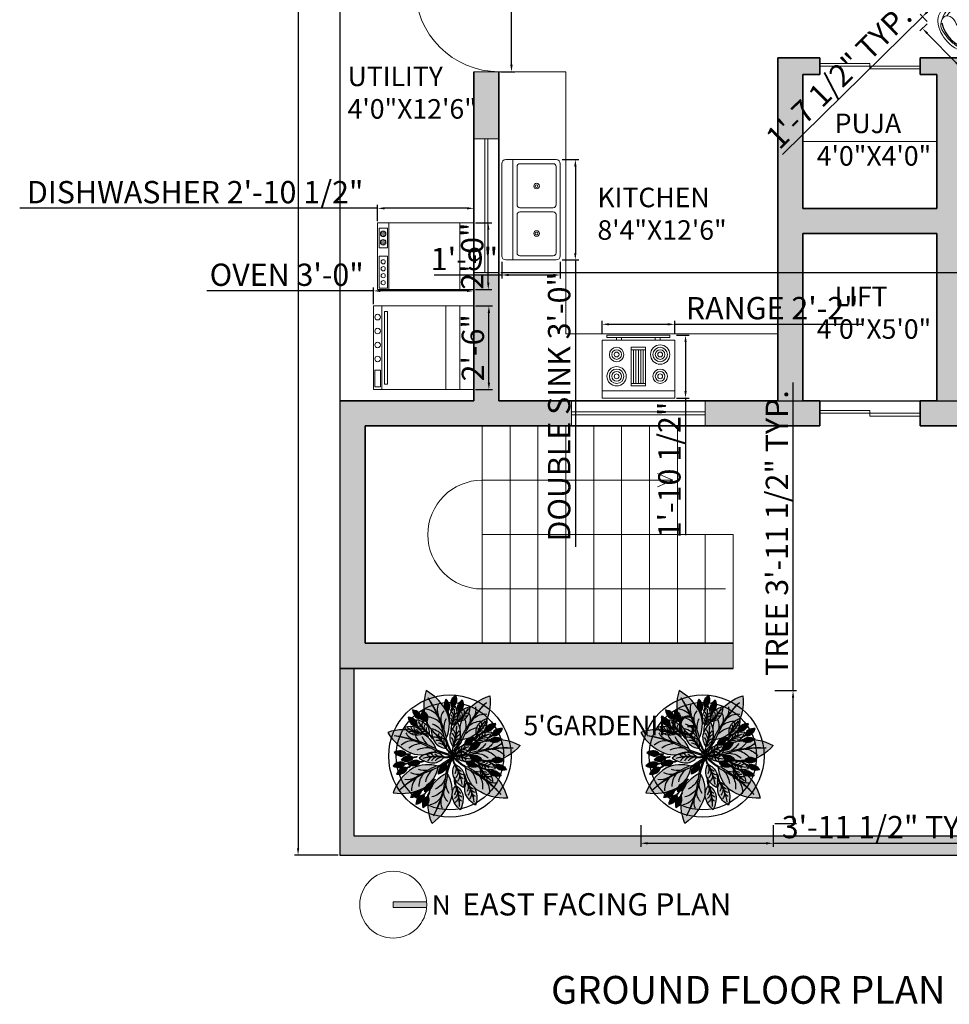
# Model space of a CAD drawing. Units: inches. Extents: x 2700 to 4052, y 1030 to 1872.
# Tile 1 of 8: x 2700 to 3033, y 1048 to 1401. Entities that reach past the tile are written whole.
import ezdxf

# ---------------------------------------------------------------- set-up
doc = ezdxf.new("R2010")
doc.units = ezdxf.units.IN
for name, color, linetype, lineweight in [('A-ANNO-DIMS', 2, 'Continuous', 13), ('A-ANNO-SYMB', 7, 'Continuous', 18), ('A-ANNO-TITL', 7, 'Continuous', 25), ('A-AREA-IDEN', 7, 'Continuous', 18), ('A-DOOR', 4, 'Continuous', 18), ('A-EQPM', 8, 'Continuous', 18), ('A-FLOR-CASE', 8, 'Continuous', 18), ('A-FLOR-FIXT', 9, 'Continuous', 18), ('A-FLOR-STRS', 7, 'Continuous', 18), ('A-FURN', 8, 'Continuous', 18), ('A-GLAZ', 4, 'Continuous', 18), ('A-WALL', 7, 'Continuous', 35), ('A-WALL-PATT', 7, 'Continuous', 13), ('C-PROP', 7, 'Continuous', 25), ('L-PLNT', 3, 'Continuous', 13)]:
    doc.layers.add(name, color=color, linetype=linetype, lineweight=lineweight)
doc.layers.add('C-SITE-PATT', color=252, linetype='Continuous', lineweight=13, true_color=0x939598)
doc.layers.add('IFF-FURN-DETAIL', color=250, linetype='Continuous')
doc.layers.add('MESA', color=7, linetype='Continuous')
doc.styles.get("Standard").update_dxf_attribs({"font": 'arial.ttf'})
doc.dimstyles.new('ISO-25', dxfattribs={"dimtxt": 8, "dimasz": 2.5, "dimexe": 1.25, "dimexo": 0.625, "dimtad": 1, "dimdec": 1, "dimlunit": 3, "dimtxsty": 'Standard', "dimcen": 2.5, "dimclrt": 1, "dimadec": 0, "dimazin": 0, "dimtfac": 1, "dimtdec": 1, "dimtmove": 0, "dimatfit": 3, "dimfxl": 1, "dimarcsym": 0})

# ---------------------------------------------------------------- blocks, each defined once
blk = doc.blocks.new('ILNG95')
for points in [[(120, 308, -0.32971), (51, 384, -0.036099), (50, 422, -0.497733), (75, 439, -0.070621), (96, 429, 0.101868), (133, 414, 0.091794), (259, 412, 0.024114), (351, 433, -0.090294), (638, 458, -0.132412), (775, 407, -0.068618), (816, 368, -0.184346), (943, 0, 1.803905)], [(120, 308, 0.138132), (244, 313, 0.001085), (325, 339, -0.034227), (462, 375, -0.033255), (567, 387, -0.137428), (727, 350, -4.561553)], [(120, 308, 0.138132), (244, 313, 0.001085), (325, 339, -0.034227), (462, 375, -0.033255), (567, 387, -0.137428), (727, 350, -4.561553)], [(235, 308, 0.064243), (394, 307, 0.04414), (433, 315, -0.118032), (643, 329, -6.296816)], [(235, 308, 0.064243), (394, 307, 0.04414), (433, 315, -0.118032), (643, 329, -6.296816)], [(639, 0, 0.078302), (612, 161, -0.233633), (633, 315, -0.28763), (710, 349, -0.317923), (875, 193, -0.032882), (900, 0, 1.140397)], [(639, 0, 0.078302), (612, 161, -0.233633), (633, 315, -0.28763), (710, 349, -0.317923), (875, 193, -0.032882), (900, 0, 1.140397)], [(120, -308, 0.32971), (51, -384, 0.036099), (50, -422, 0.497733), (75, -439, 0.070621), (96, -429, -0.101868), (133, -414, -0.091794), (259, -412, -0.024114), (351, -433, 0.090294), (638, -458, 0.132412), (775, -407, 0.068618), (816, -368, 0.184346), (943, 0, -1.803905)], [(639, 0, -0.078302), (612, -161, 0.233633), (633, -315, 0.28763), (710, -349, 0.317923), (875, -193, 0.032882), (900, 0, -1.140397)], [(639, 0, -0.078302), (612, -161, 0.233633), (633, -315, 0.28763), (710, -349, 0.317923), (875, -193, 0.032882), (900, 0, -1.140397)], [(120, -308, -0.138132), (244, -313, -0.001085), (325, -339, 0.034227), (462, -375, 0.033255), (567, -387, 0.137428), (727, -350, 4.561553)], [(120, -308, -0.138132), (244, -313, -0.001085), (325, -339, 0.034227), (462, -375, 0.033255), (567, -387, 0.137428), (727, -350, 4.561553)], [(235, -308, -0.064243), (394, -307, -0.04414), (433, -315, 0.118032), (643, -329, 6.296816)], [(235, -308, -0.064243), (394, -307, -0.04414), (433, -315, 0.118032), (643, -329, 6.296816)]]:
    blk.add_lwpolyline(points, format="xyb")
blk.add_arc((759, 1), 709, 154.3281, 205.801)
at = {"layer": 'IFF-FURN-DETAIL'}
blk.add_arc((326, -2), 549, 326.8997, 34.6691, dxfattribs=at)
blk.add_arc((326, -2), 549, 326.8997, 34.6691, dxfattribs=at)
blk = doc.blocks.new('Range-Oven - 30 in top')
for p, q in [((0, -3), (30, -3)), ((12, -6), (18, -6)), ((13, -20), (13, -6)), ((14, -6), (14, -20)), ((15, -20), (15, -6)), ((16, -6), (16, -20)), ((17, -20), (17, -6)), ((18, -20), (12, -20)), ((6, -24), (6, -25)), ((8, -25), (8, -24)), ((22, -25), (22, -24)), ((24, -24), (24, -25))]:
    blk.add_line(p, q)
for points in [[(0, -24), (0, 0), (30, 0), (30, -24)], [(12, -21), (12, -5), (18, -5), (18, -21)], [(2, -26), (2, -25), (28, -25), (28, -26)]]:
    blk.add_lwpolyline(points, close=True)
for centre, radius in [((6, -9), 4), ((6, -9), 3), ((6, -9), 2), ((6, -9), 1), ((24, -9), 3), ((24, -9), 2), ((24, -9), 1), ((6, -18), 3), ((6, -18), 2), ((24, -18), 4), ((24, -18), 3), ((24, -18), 2), ((6, -18), 1), ((24, -18), 1)]:
    blk.add_circle(centre, radius)
blk = doc.blocks.new('Sink-double - 36 in top')
for p, q in [((-18, -4), (18, -4)), ((-0.75, -18.5), (-0.75, -6.5)), ((0.75, -6.5), (0.75, -18.5))]:
    blk.add_line(p, q)
for points in [[(-16.5, 0), (16.5, 0)], [(-18, -19.5), (-18, -1.5)], [(18, -1.5), (18, -19.5)], [(-16.5, -18.5), (-16.5, -6.5)], [(-15.5, -5.5), (-1.75, -5.5)], [(1.75, -5.5), (15.5, -5.5)], [(16.5, -6.5), (16.5, -18.5)], [(16.5, -21), (-16.5, -21)], [(-1.75, -19.5), (-15.5, -19.5)], [(15.5, -19.5), (1.75, -19.5)]]:
    blk.add_lwpolyline(points)
for centre, radius in [((-8.5, -12.5), 1), ((-8.5, -12.5), 0.5), ((8.5, -12.5), 1), ((8.5, -12.5), 0.5)]:
    blk.add_circle(centre, radius)
for centre, radius, start, end in [((-16.5, -1.5), 1.5, 90, 180), ((16.5, -1.5), 1.5, 0, 90), ((-15.5, -6.5), 1, 90, 180), ((-1.75, -6.5), 1, 0, 90), ((1.75, -6.5), 1, 90, 180), ((15.5, -6.5), 1, 0, 90), ((-16.5, -19.5), 1.5, 180, 270), ((-15.5, -18.5), 1, 180, 270), ((-1.75, -18.5), 1, 270, 0), ((1.75, -18.5), 1, 180, 270), ((15.5, -18.5), 1, 270, 0), ((16.5, -19.5), 1.5, 270, 0)]:
    blk.add_arc(centre, radius, start, end)
blk = doc.blocks.new('Range-Oven - 30 in front')
for p, q in [((0, 33.00005), (30, 33.00005)), ((30, 10), (0, 10)), ((0, 5), (30, 5))]:
    blk.add_line(p, q)
for points in [[(0, 0), (0, 36.00005), (30, 36.00005), (30, 0)], [(1, 33.50005), (1, 35.50005), (7, 35.50005), (7, 33.50005)], [(2, 31.00005), (2, 32.00005), (28, 32.00005), (28, 31.00005)]]:
    blk.add_lwpolyline(points, close=True)
for centre in [(11, 34.50005), (16, 34.50005), (21, 34.50005), (26, 34.50005)]:
    blk.add_circle(centre, 1)
blk = doc.blocks.new('Dishwasher')
for p, q in [((16, 32.5), (16.75, 32.5)), ((16.5, 32), (16.2942, 31.7942)), ((16.3156, 33.1843), (16.5, 33)), ((17, 32.75), (17, 33.5)), ((17, 32.25), (17, 31.5)), ((18, 32.5), (17.25, 32.5)), ((17.5, 33), (17.6938, 33.1938)), ((17.7061, 31.7939), (17.5, 32)), ((19, 32.5), (19.75, 32.5)), ((19.5, 32), (19.2942, 31.7942)), ((19.3156, 33.1843), (19.5, 33)), ((20, 32.75), (20, 33.5)), ((20, 32.25), (20, 31.5)), ((21, 32.5), (20.25, 32.5)), ((20.5, 33), (20.6938, 33.1938)), ((20.7061, 31.7939), (20.5, 32)), ((24, 30.5), (0, 30.5)), ((0, 5), (24, 5))]:
    blk.add_line(p, q)
for points in [[(0, 0), (0, 34.5), (24, 34.5), (24, 0)], [(0.5, 31), (0.5, 34), (12, 34), (12, 31)], [(15, 31), (15, 34), (22, 34), (22, 31)]]:
    blk.add_lwpolyline(points, close=True)
for centre, radius in [((2.5, 32.5), 0.75), ((5, 32.5), 0.75), ((7.5, 32.5), 0.75), ((10, 32.5), 0.75), ((17, 32.5), 1), ((20, 32.5), 1)]:
    blk.add_circle(centre, radius)
blk = doc.blocks.new('folha Ant')
at = {"layer": 'MESA', "ltscale": 0.8}
h = blk.add_hatch(color=256, dxfattribs=at)
h.dxf.hatch_style = 1
h.set_gradient(color1=(103, 159, 96), color2=(179, 207, 175), one_color=1, tint=0.75, name='INVCURVED')
h.paths.add_polyline_path([(0.2266, 0.0676, 0.199512), (0.0989, 0.0067, 0.09675), (0.3533, 0.0075, -0.086654), (0.1023, -0.0053, 0.192489), (0.2266, -0.0624, 0.158608), (0.3953, 0.0026, 0.158608)])
h = blk.add_hatch(color=256, dxfattribs=at)
h.dxf.hatch_style = 1
h.set_gradient(color1=(179, 116, 77), color2=(114, 74, 49), one_color=1, tint=0.32, name='CURVED')
h.paths.add_polyline_path([(0.05, -0.0003), (0.0485, 0.0057, 0.033108), (0, 0, 0.809082), (0.002, -0.006, -0.032777)])
h.paths.add_polyline_path([(0.0973, 0.0049, 0.033108), (0.0485, 0.0057), (0.05, -0.0003, -0.032777), (0.0983, -0.001), (0.0953, 0.0026)])
h = blk.add_hatch(color=256, dxfattribs=at)
h.dxf.hatch_style = 1
h.set_gradient(color1=(103, 159, 96), color2=(52, 80, 48), one_color=1, tint=0.25)
h.paths.add_polyline_path([(0.3533, 0.0075, -0.09675), (0.0989, 0.0067, 0.007527), (0.0953, 0.0026, 0.014292), (0.1023, -0.0053, 0.086654)])
blk.add_lwpolyline([(0.0983, -0.001), (0.0953, 0.0026), (0.0973, 0.0049, 0.066288), (0, 0, 0.809082), (0.002, -0.006, -0.065625)], format="xyb", close=True, dxfattribs=at)
for centre, radius, start, end in [((0.2359, -0.1164), 0.1842, 92.9121, 139.7695), ((0.211, -0.2242), 0.2922, 50.9055, 86.9554), ((0.2359, 0.1215), 0.1842, 220.2305, 267.0879), ((0.2242, 0.6583), 0.6635, 259.119, 281.2235), ((0.1912, 0.7199), 0.7306, 263.0097, 282.8199), ((0.1144, 0.1192), 0.1187, 277.6411, 318.482), ((0.1515, 0.1013), 0.1129, 290.5634, 330.4539), ((0.211, 0.2293), 0.2922, 273.0446, 309.0945), ((0.2123, 0.0879), 0.0955, 283.0013, 333.1911), ((0.1127, -0.1239), 0.1214, 41.7528, 70.1061), ((0.1853, -0.0821), 0.0727, 27.7376, 79.2347), ((0.2381, -0.0995), 0.0902, 48.8027, 88.011)]:
    blk.add_arc(centre, radius, start, end, dxfattribs=at)
blk = doc.blocks.new('arvore L')
at = {"layer": 'MESA', "ltscale": 0.8}
for radius in [0.35, 0.3077]:
    blk.add_circle((-0.0174, -0.0123), radius, dxfattribs=at)
at = {"layer": 'MESA'}
for p, rotation in [((-0.0038, -0.0034), 111.8634939329907), ((-0.0015, -0.0116), 159.7023978146411), ((-0.002, -0.0223), 210.0932896211622)]:
    blk.add_blockref('folha Ant', p, dxfattribs=dict(at, rotation=rotation))
at = {"layer": 'MESA', "xscale": -1}
for p, rotation in [((-0.0038, 0.0015), 237.4553048776787), ((-0.0054, -0.0158), 189.5771815307885), ((-0.0065, -0.0187), 73.74235818062448), ((-0.0036, -0.0152), 143.2116612097536)]:
    blk.add_blockref('folha Ant', p, dxfattribs=dict(at, rotation=rotation))
at = {"layer": 'MESA'}
for p, xscale, yscale, zscale, rotation in [((-0.0106, 0.2458), -0.2372171158460138, 0.2372171158460219, 0.2372171158460401, 254.670727296299), ((-0.0228, 0.2207), 0.2372171158460145, 0.2372171158460145, 0.2372171158460145, 100.7442899234288), ((0.0048, 0.1582), 0.3672988726102984, 0.3672988726102984, 0.3672988726102984, 49.45009658216958), ((0.0276, 0.2187), -0.2372171158460138, 0.2372171158460219, 0.2372171158460401, 254.670727296299), ((-0.1648, 0.1856), 0.2372171158460308, 0.2372171158460308, 0.2372171158460308, 134.9461414081513), ((-0.1441, 0.1612), -0.2372171158460326, 0.2372171158460219, 0.2372171158460401, 288.8725787810177), ((-0.0127, 0.1293), 0.367298872610303, 0.367298872610303, 0.367298872610303, 78.9591877781593), ((-0.1408, 0.1026), -0.3672988726103232, 0.3672988726103199, 0.3672988726103326, 340.1667721222815), ((-0.189, 0.1454), 0.2372171158460308, 0.2372171158460308, 0.2372171158460308, 134.9461414081513), ((-0.1144, 0.0854), -0.3672988726103342, 0.3672988726103199, 0.3672988726103326, 310.6576809262878), ((-0.0068, -0.0029), 0.4722192998870434, 0.4722192998870434, 0.4722192998870434, 78.95918777814883), ((0.1186, 0.0777), -0.3672988726103297, 0.3672988726103199, 0.3672988726103326, 240.0025576387842), ((0.1681, 0.1193), 0.2372171158460773, 0.2372171158460773, 0.2372171158460773, 34.78192692463861), ((-0.0091, -0.003), 0.4722192998870449, 0.4722192998870449, 0.4722192998870449, 127.7597565182155), ((0.0972, 0.0516), -0.3672988726102771, 0.3672988726103199, 0.3672988726103326, 210.4934664427891), ((0.2063, 0.0923), 0.2372171158460773, 0.2372171158460773, 0.2372171158460773, 34.78192692463861), ((-0.0206, -0.0213), -0.3672988726102771, 0.3672988726103199, 0.3672988726103326, 210.4934664427891), ((0.0473, 0.041), 0.2372171158460773, 0.2372171158460773, 0.2372171158460773, 34.78192692463861), ((0.0807, 0.0116), 0.2372171158460773, 0.2372171158460773, 0.2372171158460773, 34.78192692463861), ((0.1867, 0.0725), -0.237217115846069, 0.2372171158460219, 0.2372171158460401, 188.7083642975024), ((-0.2438, -0.0026), 0.2372171158460885, 0.2372171158460885, 0.2372171158460885, 173.1881796188063), ((-0.0061, -0.0164), 0.4722192998870134, 0.4722192998870134, 0.4722192998870134, 181.8145453364702), ((-0.0239, 0.0106), 0.3672988726102808, 0.3672988726102808, 0.3672988726102808, 341.2516722292817), ((0.082, -0.001), -0.2372171158460231, 0.2372171158460219, 0.2372171158460401, 156.9632117474216), ((-0.2506, -0.0512), 0.2372171158460153, 0.2372171158460153, 0.2372171158460153, 190.4360105724469), ((-0.241, -0.0679), 0.237217115846034, 0.237217115846034, 0.237217115846034, 209.7732768087273), ((-0.2046, -0.0159), 0.2372171158460153, 0.2372171158460153, 0.2372171158460153, 190.4360105724469), ((-0.1644, -0.0415), 0.2372171158460153, 0.2372171158460153, 0.2372171158460153, 190.4360105724469), ((-0.024, -0.0418), -0.2372171158460388, 0.2372171158460219, 0.2372171158460401, 51.68033384933957), ((-0.0047, -0.0173), -0.4722192998870682, 0.4722192998870583, 0.4722192998870367, 110.7618316866296), ((0.0552, -0.0366), -0.2372171158460231, 0.2372171158460219, 0.2372171158460401, 156.9632117474216), ((0.1063, -0.0368), 0.3672988726102808, 0.3672988726102808, 0.3672988726102808, 341.2516722292817), ((0.1326, -0.058), 0.3672988726103005, 0.3672988726103005, 0.3672988726103005, 311.7425810332929), ((0.1982, -0.0391), 0.2372171158460078, 0.2372171158460078, 0.2372171158460078, 3.036774374557308), ((0.2214, -0.0544), -0.2372171158460231, 0.2372171158460219, 0.2372171158460401, 156.9632117474216), ((0.0645, -0.1182), -0.4722192998870682, 0.4722192998870583, 0.4722192998870367, 110.7618316866296), ((0.1895, -0.0887), -0.2372171158460231, 0.2372171158460219, 0.2372171158460401, 156.9632117474216), ((-0.1025, -0.1443), -0.2372171158460388, 0.2372171158460219, 0.2372171158460401, 51.68033384933957), ((0.0082, -0.1357), -0.4722192998870255, 0.4722192998870583, 0.4722192998870367, 100.6603657106226), ((-0.1617, -0.1996), -0.2372171158460624, 0.2372171158460219, 0.2372171158460401, 32.34306761306672), ((-0.1514, -0.2159), -0.2372171158460388, 0.2372171158460219, 0.2372171158460401, 51.68033384933957), ((-0.1351, -0.2206), -0.2372171158460438, 0.2372171158460219, 0.2372171158460401, 68.92816480300668)]:
    blk.add_blockref('folha Ant', p, dxfattribs=dict(at, xscale=xscale, yscale=yscale, zscale=zscale, rotation=rotation))
blk = doc.blocks.new('*D20')
at = {"layer": 'A-ANNO-DIMS', "color": 0, "lineweight": -2, "transparency": 16777216}
for p, q in [((2814.04, 1821.52), (2798.4, 1821.52)), ((2799.65, 1819.02), (2799.65, 1104.02)), ((2814.04, 1101.52), (2798.4, 1101.52))]:
    blk.add_line(p, q, dxfattribs=at)
at = {"layer": 'A-ANNO-DIMS', "color": 0, "transparency": 16777216}
for points in [[(2799.23, 1819.02), (2800.06, 1819.02), (2799.65, 1821.52)], [(2799.23, 1104.02), (2800.06, 1104.02), (2799.65, 1101.52)]]:
    blk.add_solid(points, dxfattribs=at)
at = {"layer": 'Defpoints', "color": 0, "transparency": 16777216}
for p in [(2814.67, 1821.52), (2799.65, 1101.52), (2814.67, 1101.52)]:
    blk.add_point(p, dxfattribs=at)
at = {"layer": 'A-ANNO-DIMS', "color": 0, "transparency": 16777216, "insert": (2794.94, 1461.52), "char_height": 8, "attachment_point": 5, "rotation": 90}
blk.add_mtext("60'", dxfattribs=at)
blk = doc.blocks.new('DOOR-SWING-30IN')
for p, q in [((-1, 30), (-1, 0)), ((0, 30), (0, 0)), ((0, 0), (-1, 0))]:
    blk.add_line(p, q)
blk.add_arc((0, 0), 30, 90, 180)
blk = doc.blocks.new('DOOR-SLIDING-36IN')
for p, q in [((18, 2), (0, 2)), ((36, 1), (0, 1)), ((18, 2), (18, 0)), ((36, 0), (18, 0))]:
    blk.add_line(p, q)
blk = doc.blocks.new('WINDOW-48IN')
for p, q in [((-24, -4.5), (-24, 4.5)), ((24, -4.5), (24, 4.5)), ((-24, 0.5), (24, 0.5)), ((-24, -0.5), (24, -0.5))]:
    blk.add_line(p, q)
blk = doc.blocks.new('STAIR-RETURN-FLIGHT')
for p, q in [((19.5, 87), (19.5, 9)), ((29.5, 87), (29.5, 9)), ((39.5, 87), (39.5, 9)), ((49.5, 87), (49.5, 9)), ((59.5, 87), (59.5, 9)), ((69.5, 87), (69.5, 9)), ((79.5, 87), (79.5, 9)), ((89.5, 87), (89.5, 9)), ((87.91, 67.5), (82.37, 69.91)), ((87.91, 67.5), (82.37, 65.09)), ((109.5, 48), (19.5, 48)), ((99.5, 48), (99.5, 9)), ((109.5, 48), (109.5, 0))]:
    blk.add_line(p, q)
blk.add_lwpolyline([(106.75, 28.5), (19.5, 28.5, -1), (19.5, 67.5), (87.91, 67.5)], format="xyb")
blk = doc.blocks.new('NORTH-INDICATOR')
at = {"transparency": 33554687}
h = blk.add_hatch(color=256, dxfattribs=at)
h.dxf.hatch_style = 1
h.paths.add_polyline_path([(0, 1), (0, -1), (11.96, -1, 0.020861), (12, 0, 0.020861), (11.96, 1)])
for p, q in [((0, -1), (0, 1)), ((0, 1), (11.96, 1)), ((12, -1), (0, -1))]:
    blk.add_line(p, q)
blk.add_circle((0, 0), 12)
blk.add_text('N', height=6.9).set_placement((13.83, -3.53))
blk = doc.blocks.new('*D72')
at = {"layer": 'A-ANNO-DIMS', "color": 0, "lineweight": -2, "transparency": 16777216}
for p, q in [((2876.17, 1412.52), (2876.17, 1542.6)), ((2872.29, 1412.52), (2877.42, 1412.52)), ((2876.17, 1385.02), (2876.17, 1410.02)), ((2872.29, 1382.52), (2877.42, 1382.52))]:
    blk.add_line(p, q, dxfattribs=at)
at = {"layer": 'A-ANNO-DIMS', "color": 0, "transparency": 16777216}
for points in [[(2875.75, 1410.02), (2876.59, 1410.02), (2876.17, 1412.52)], [(2875.75, 1385.02), (2876.59, 1385.02), (2876.17, 1382.52)]]:
    blk.add_solid(points, dxfattribs=at)
at = {"layer": 'Defpoints', "color": 0, "transparency": 16777216}
for p in [(2871.67, 1412.52), (2876.17, 1412.52), (2871.67, 1382.52)]:
    blk.add_point(p, dxfattribs=at)
at = {"layer": 'A-ANNO-DIMS', "color": 1, "transparency": 16777216, "insert": (2871.41, 1478.81), "char_height": 8, "attachment_point": 5, "rotation": 90}
blk.add_mtext('SWING DOOR 2\'-6" TYP.', dxfattribs=at)
blk = doc.blocks.new('*D82')
at = {"layer": 'A-ANNO-DIMS', "color": 0, "lineweight": -2, "transparency": 16777216}
for p, q in [((3025.17, 1399.72), (3022.61, 1397.19)), ((3025.25, 1396.29), (3035.65, 1385.75)), ((3039.07, 1385.62), (3036.51, 1383.09)), ((3037.4, 1383.97), (3100.81, 1319.68))]:
    blk.add_line(p, q, dxfattribs=at)
at = {"layer": 'A-ANNO-DIMS', "color": 0, "transparency": 16777216}
for points in [[(3025.55, 1396.58), (3024.96, 1396), (3023.5, 1398.07)], [(3035.95, 1386.04), (3035.35, 1385.46), (3037.4, 1383.97)]]:
    blk.add_solid(points, dxfattribs=at)
at = {"layer": 'Defpoints', "color": 0, "transparency": 16777216}
for p in [(3025.61, 1400.16), (3039.52, 1386.06), (3037.4, 1383.97)]:
    blk.add_point(p, dxfattribs=at)
at = {"layer": 'A-ANNO-DIMS', "color": 1, "transparency": 16777216, "insert": (3073.38, 1354.28), "char_height": 8, "attachment_point": 5, "rotation": 314.6051}
blk.add_mtext('CHAIR 1\'-8" TYP.', dxfattribs=at)
blk = doc.blocks.new('*D83')
at = {"layer": 'A-ANNO-DIMS', "color": 0, "lineweight": -2, "transparency": 16777216}
for p, q in [((3039.09, 1414.33), (3036.56, 1416.89)), ((3035.66, 1414.24), (3025.31, 1404.03)), ((3023.53, 1402.27), (2973.4, 1352.84)), ((3025.17, 1400.6), (3022.65, 1403.16))]:
    blk.add_line(p, q, dxfattribs=at)
at = {"layer": 'A-ANNO-DIMS', "color": 0, "transparency": 16777216}
for points in [[(3035.37, 1414.54), (3035.95, 1413.94), (3037.44, 1416)], [(3025.01, 1404.33), (3025.6, 1403.73), (3023.53, 1402.27)]]:
    blk.add_solid(points, dxfattribs=at)
at = {"layer": 'Defpoints', "color": 0, "transparency": 16777216}
for p in [(3039.52, 1413.88), (3023.53, 1402.27), (3025.61, 1400.16)]:
    blk.add_point(p, dxfattribs=at)
at = {"layer": 'A-ANNO-DIMS', "color": 1, "transparency": 16777216, "insert": (2994.23, 1380.07), "char_height": 8, "attachment_point": 5, "rotation": 44.6051}
blk.add_mtext('1\'-7 1/2" TYP.', dxfattribs=at)
blk = doc.blocks.new('*D88')
at = {"layer": 'A-ANNO-DIMS', "color": 0, "lineweight": -2, "transparency": 16777216}
for p, q in [((2977.13, 1160.56), (2977.13, 1271.05)), ((2970.61, 1160.56), (2978.38, 1160.56)), ((2977.13, 1115.44), (2977.13, 1158.06)), ((2970.61, 1112.94), (2978.38, 1112.94))]:
    blk.add_line(p, q, dxfattribs=at)
at = {"layer": 'A-ANNO-DIMS', "color": 0, "transparency": 16777216}
for points in [[(2976.71, 1158.06), (2977.54, 1158.06), (2977.13, 1160.56)], [(2976.71, 1115.44), (2977.54, 1115.44), (2977.13, 1112.94)]]:
    blk.add_solid(points, dxfattribs=at)
at = {"layer": 'Defpoints', "color": 0, "transparency": 16777216}
for p in [(2969.98, 1160.56), (2977.13, 1160.56), (2969.98, 1112.94)]:
    blk.add_point(p, dxfattribs=at)
at = {"layer": 'A-ANNO-DIMS', "color": 1, "transparency": 16777216, "insert": (2972.36, 1217.06), "char_height": 8, "attachment_point": 5, "rotation": 90}
blk.add_mtext('TREE 3\'-11 1/2" TYP.', dxfattribs=at)
blk = doc.blocks.new('*D89')
at = {"layer": 'A-ANNO-DIMS', "color": 0, "lineweight": -2, "transparency": 16777216}
for p, q in [((2922.49, 1112.32), (2922.49, 1104.55)), ((2969.98, 1112.32), (2969.98, 1104.55)), ((2924.99, 1105.8), (2967.48, 1105.8)), ((2969.98, 1105.8), (3047.35, 1105.8))]:
    blk.add_line(p, q, dxfattribs=at)
at = {"layer": 'A-ANNO-DIMS', "color": 0, "transparency": 16777216}
for points in [[(2924.99, 1106.22), (2924.99, 1105.38), (2922.49, 1105.8)], [(2967.48, 1106.22), (2967.48, 1105.38), (2969.98, 1105.8)]]:
    blk.add_solid(points, dxfattribs=at)
at = {"layer": 'Defpoints', "color": 0, "transparency": 16777216}
for p in [(2922.49, 1112.94), (2969.98, 1112.94), (2969.98, 1105.8)]:
    blk.add_point(p, dxfattribs=at)
at = {"layer": 'A-ANNO-DIMS', "color": 1, "transparency": 16777216, "insert": (3009.92, 1110.57), "char_height": 8, "attachment_point": 5}
blk.add_mtext('3\'-11 1/2" TYP.', dxfattribs=at)
blk = doc.blocks.new('*D94')
at = {"layer": 'A-ANNO-DIMS', "color": 0, "lineweight": -2, "transparency": 16777216}
for p, q in [((2908.66, 1288.66), (2908.66, 1293.19)), ((2934.68, 1288.66), (2934.68, 1293.19)), ((2911.16, 1291.94), (2932.18, 1291.94)), ((2934.68, 1291.94), (3002.13, 1291.94))]:
    blk.add_line(p, q, dxfattribs=at)
at = {"layer": 'A-ANNO-DIMS', "color": 0, "transparency": 16777216}
for points in [[(2911.16, 1292.36), (2911.16, 1291.52), (2908.66, 1291.94)], [(2932.18, 1292.36), (2932.18, 1291.52), (2934.68, 1291.94)]]:
    blk.add_solid(points, dxfattribs=at)
at = {"layer": 'Defpoints', "color": 0, "transparency": 16777216}
for p in [(2934.68, 1291.94), (2908.66, 1288.04), (2934.68, 1288.04)]:
    blk.add_point(p, dxfattribs=at)
at = {"layer": 'A-ANNO-DIMS', "color": 1, "transparency": 16777216, "insert": (2969.65, 1296.7), "char_height": 8, "attachment_point": 5}
blk.add_mtext('RANGE 2\'-2"', dxfattribs=at)
blk = doc.blocks.new('*D95')
at = {"layer": 'A-ANNO-DIMS', "color": 0, "lineweight": -2, "transparency": 16777216}
for p, q in [((2935.3, 1288.04), (2939.83, 1288.04)), ((2938.58, 1285.54), (2938.58, 1267.99)), ((2935.3, 1265.49), (2939.83, 1265.49)), ((2938.58, 1265.49), (2938.58, 1216.37))]:
    blk.add_line(p, q, dxfattribs=at)
at = {"layer": 'A-ANNO-DIMS', "color": 0, "transparency": 16777216}
for points in [[(2938.17, 1285.54), (2939, 1285.54), (2938.58, 1288.04)], [(2938.17, 1267.99), (2939, 1267.99), (2938.58, 1265.49)]]:
    blk.add_solid(points, dxfattribs=at)
at = {"layer": 'Defpoints', "color": 0, "transparency": 16777216}
for p in [(2934.68, 1288.04), (2934.68, 1265.49), (2938.58, 1265.49)]:
    blk.add_point(p, dxfattribs=at)
at = {"layer": 'A-ANNO-DIMS', "color": 1, "transparency": 16777216, "insert": (2933.82, 1239.68), "char_height": 8, "attachment_point": 5, "rotation": 90}
blk.add_mtext('1\'-10 1/2"', dxfattribs=at)
blk = doc.blocks.new('*D96')
at = {"layer": 'A-ANNO-DIMS', "color": 0, "lineweight": -2, "transparency": 16777216}
for p, q in [((2894.29, 1351.02), (2900.32, 1351.02)), ((2899.07, 1348.52), (2899.07, 1317.52)), ((2894.29, 1315.02), (2900.32, 1315.02)), ((2899.07, 1315.02), (2899.07, 1212.15))]:
    blk.add_line(p, q, dxfattribs=at)
at = {"layer": 'A-ANNO-DIMS', "color": 0, "transparency": 16777216}
for points in [[(2898.65, 1348.52), (2899.49, 1348.52), (2899.07, 1351.02)], [(2898.65, 1317.52), (2899.49, 1317.52), (2899.07, 1315.02)]]:
    blk.add_solid(points, dxfattribs=at)
at = {"layer": 'Defpoints', "color": 0, "transparency": 16777216}
for p in [(2893.67, 1351.02), (2893.67, 1315.02), (2899.07, 1315.02)]:
    blk.add_point(p, dxfattribs=at)
at = {"layer": 'A-ANNO-DIMS', "color": 1, "transparency": 16777216, "insert": (2894.3, 1262.34), "char_height": 8, "attachment_point": 5, "rotation": 90}
blk.add_mtext('DOUBLE SINK 3\'-0"', dxfattribs=at)
blk = doc.blocks.new('*D97')
at = {"layer": 'A-ANNO-DIMS', "color": 0, "lineweight": -2, "transparency": 16777216}
for p, q in [((2872.67, 1314.4), (2872.67, 1308.37)), ((2893.67, 1314.4), (2893.67, 1308.37)), ((2872.67, 1309.62), (2848.41, 1309.62)), ((2891.17, 1309.62), (2875.17, 1309.62))]:
    blk.add_line(p, q, dxfattribs=at)
at = {"layer": 'A-ANNO-DIMS', "color": 0, "transparency": 16777216}
for points in [[(2875.17, 1310.04), (2875.17, 1309.21), (2872.67, 1309.62)], [(2891.17, 1310.04), (2891.17, 1309.21), (2893.67, 1309.62)]]:
    blk.add_solid(points, dxfattribs=at)
at = {"layer": 'Defpoints', "color": 0, "transparency": 16777216}
for p in [(2872.67, 1315.02), (2893.67, 1315.02), (2872.67, 1309.62)]:
    blk.add_point(p, dxfattribs=at)
at = {"layer": 'A-ANNO-DIMS', "color": 1, "transparency": 16777216, "insert": (2859.29, 1314.33), "char_height": 8, "attachment_point": 5}
blk.add_mtext('1\'-9"', dxfattribs=at)
blk = doc.blocks.new('*D98')
at = {"layer": 'A-ANNO-DIMS', "color": 0, "lineweight": -2, "transparency": 16777216}
for p, q in [((2826.67, 1303.92), (2766.95, 1303.92)), ((2826.67, 1299.14), (2826.67, 1305.17)), ((2860.17, 1303.92), (2829.17, 1303.92)), ((2862.67, 1299.14), (2862.67, 1305.17))]:
    blk.add_line(p, q, dxfattribs=at)
at = {"layer": 'A-ANNO-DIMS', "color": 0, "transparency": 16777216}
for points in [[(2829.17, 1304.33), (2829.17, 1303.5), (2826.67, 1303.92)], [(2860.17, 1304.33), (2860.17, 1303.5), (2862.67, 1303.92)]]:
    blk.add_solid(points, dxfattribs=at)
at = {"layer": 'Defpoints', "color": 0, "transparency": 16777216}
for p in [(2826.67, 1303.92), (2826.67, 1298.52), (2862.67, 1298.52)]:
    blk.add_point(p, dxfattribs=at)
at = {"layer": 'A-ANNO-DIMS', "color": 1, "transparency": 16777216, "insert": (2795.56, 1308.68), "char_height": 8, "attachment_point": 5}
blk.add_mtext('OVEN 3\'-0"', dxfattribs=at)
blk = doc.blocks.new('*D99')
at = {"layer": 'A-ANNO-DIMS', "color": 0, "lineweight": -2, "transparency": 16777216}
for p, q in [((2863.29, 1298.52), (2869.32, 1298.52)), ((2868.07, 1271.02), (2868.07, 1296.02)), ((2863.29, 1268.52), (2869.32, 1268.52))]:
    blk.add_line(p, q, dxfattribs=at)
at = {"layer": 'A-ANNO-DIMS', "color": 0, "transparency": 16777216}
for points in [[(2867.65, 1296.02), (2868.49, 1296.02), (2868.07, 1298.52)], [(2867.65, 1271.02), (2868.49, 1271.02), (2868.07, 1268.52)]]:
    blk.add_solid(points, dxfattribs=at)
at = {"layer": 'Defpoints', "color": 0, "transparency": 16777216}
for p in [(2862.67, 1298.52), (2868.07, 1298.52), (2862.67, 1268.52)]:
    blk.add_point(p, dxfattribs=at)
at = {"layer": 'A-ANNO-DIMS', "color": 1, "transparency": 16777216, "insert": (2863.36, 1283.52), "char_height": 8, "attachment_point": 5, "rotation": 90}
blk.add_mtext('2\'-6"', dxfattribs=at)
blk = doc.blocks.new('*D100')
at = {"layer": 'A-ANNO-DIMS', "color": 0, "lineweight": -2, "transparency": 16777216}
for p, q in [((2828.17, 1333.54), (2699.84, 1333.54)), ((2828.17, 1328.99), (2828.17, 1334.79)), ((2860.17, 1333.54), (2830.67, 1333.54)), ((2862.67, 1328.99), (2862.67, 1334.79))]:
    blk.add_line(p, q, dxfattribs=at)
at = {"layer": 'A-ANNO-DIMS', "color": 0, "transparency": 16777216}
for points in [[(2830.67, 1333.96), (2830.67, 1333.13), (2828.17, 1333.54)], [(2860.17, 1333.96), (2860.17, 1333.13), (2862.67, 1333.54)]]:
    blk.add_solid(points, dxfattribs=at)
at = {"layer": 'Defpoints', "color": 0, "transparency": 16777216}
for p in [(2828.17, 1333.54), (2828.17, 1328.37), (2862.67, 1328.37)]:
    blk.add_point(p, dxfattribs=at)
at = {"layer": 'A-ANNO-DIMS', "color": 1, "transparency": 16777216, "insert": (2762.75, 1338.3), "char_height": 8, "attachment_point": 5}
blk.add_mtext('DISHWASHER 2\'-10 1/2"', dxfattribs=at)
blk = doc.blocks.new('*D101')
at = {"layer": 'A-ANNO-DIMS', "color": 0, "lineweight": -2, "transparency": 16777216}
for p, q in [((2863.29, 1328.37), (2869.09, 1328.37)), ((2867.84, 1306.87), (2867.84, 1325.87)), ((2863.29, 1304.37), (2869.09, 1304.37))]:
    blk.add_line(p, q, dxfattribs=at)
at = {"layer": 'A-ANNO-DIMS', "color": 0, "transparency": 16777216}
for points in [[(2867.43, 1325.87), (2868.26, 1325.87), (2867.84, 1328.37)], [(2867.43, 1306.87), (2868.26, 1306.87), (2867.84, 1304.37)]]:
    blk.add_solid(points, dxfattribs=at)
at = {"layer": 'Defpoints', "color": 0, "transparency": 16777216}
for p in [(2862.67, 1328.37), (2867.84, 1328.37), (2862.67, 1304.37)]:
    blk.add_point(p, dxfattribs=at)
at = {"layer": 'A-ANNO-DIMS', "color": 1, "transparency": 16777216, "insert": (2863.14, 1316.37), "char_height": 8, "attachment_point": 5, "rotation": 90}
blk.add_mtext('2\'-0"', dxfattribs=at)
blk = doc.blocks.new('*D114')
at = {"layer": 'A-ANNO-DIMS', "color": 0, "lineweight": -2, "transparency": 16777216}
for p, q in [((2872.29, 1310.49), (3216.52, 1310.49)), ((3215.27, 1267.02), (3215.27, 1307.99)), ((2872.29, 1264.52), (3216.52, 1264.52))]:
    blk.add_line(p, q, dxfattribs=at)
at = {"layer": 'A-ANNO-DIMS', "color": 0, "transparency": 16777216}
for points in [[(3214.85, 1307.99), (3215.69, 1307.99), (3215.27, 1310.49)], [(3214.85, 1267.02), (3215.69, 1267.02), (3215.27, 1264.52)]]:
    blk.add_solid(points, dxfattribs=at)
at = {"layer": 'Defpoints', "color": 0, "transparency": 16777216}
for p in [(2871.67, 1310.49), (3215.27, 1310.49), (2871.67, 1264.52)]:
    blk.add_point(p, dxfattribs=at)
at = {"layer": 'A-ANNO-DIMS', "color": 1, "transparency": 16777216, "insert": (3210.56, 1287.51), "char_height": 8, "attachment_point": 5, "rotation": 90}
blk.add_mtext('3\'-10"', dxfattribs=at)

msp = doc.modelspace()

# ---------------------------------------------------------------- hatches: boundary and pattern name
at = {"layer": 'A-WALL-PATT'}
h = msp.add_hatch(color=256, dxfattribs=at)
h.dxf.hatch_style = 1
h.paths.add_polyline_path([(2814.67, 1264.52), (2814.67, 1168.52), (2955.67, 1168.52), (2955.67, 1177.52), (2823.67, 1177.52), (2823.67, 1255.52), (2897.67, 1255.52), (2897.67, 1264.52), (2871.67, 1264.52), (2871.67, 1310.49), (2862.67, 1310.49), (2862.67, 1304.37), (2862.67, 1264.52)])
h.paths.add_polyline_path([(2945.67, 1255.52), (2986.67, 1255.52), (2986.67, 1264.52), (2980.67, 1264.52), (2980.67, 1324.52), (3028.67, 1324.52), (3028.67, 1264.52), (3022.67, 1264.52), (3022.67, 1255.52), (3037.67, 1255.52), (3037.67, 1378.52), (3040.67, 1378.52), (3040.67, 1387.52), (3022.67, 1387.52), (3022.67, 1381.52), (3028.67, 1381.52), (3028.67, 1333.52), (2980.67, 1333.52), (2980.67, 1381.52), (2986.67, 1381.52), (2986.67, 1387.52), (2971.67, 1387.52), (2971.67, 1264.52), (2945.67, 1264.52)])
h.paths.add_polyline_path([(2871.67, 1358.49), (2871.67, 1382.52), (2862.67, 1382.52), (2862.67, 1358.49)])
h.paths.add_polyline_path([(3091.67, 1387.52), (3088.67, 1387.52), (3088.67, 1378.52), (3091.67, 1378.52)])
h.paths.add_polyline_path([(3141.67, 1300.52), (3150.67, 1300.52), (3150.67, 1431.52), (3141.67, 1431.52), (3141.67, 1387.52), (3139.67, 1387.52), (3139.67, 1378.52), (3141.67, 1378.52)])
h.paths.add_polyline_path([(2830.28, 1565.14), (2830.28, 1604.05), (2822.03, 1604.05), (2822.03, 1565.14)], flags=9)
h.paths.add_polyline_path([(2957.35, 1565.68), (2957.35, 1611.46), (2949.11, 1611.46), (2949.11, 1565.68)], flags=9)
h.paths.add_polyline_path([(2983.54, 1697.89), (2983.54, 1743.66), (2975.29, 1743.66), (2975.29, 1697.89)], flags=9)
h.paths.add_polyline_path([(2879.08, 1800.61), (2924.85, 1800.61), (2924.85, 1808.85), (2879.08, 1808.85)], flags=9)
h.paths.add_polyline_path([(2815.49, 1361.72), (2864.45, 1361.72), (2864.45, 1388.34), (2815.49, 1388.34)], flags=9)
h.paths.add_polyline_path([(2904.6, 1318.27), (2953.91, 1318.27), (2953.91, 1344.89), (2904.6, 1344.89)], flags=9)
h.paths.add_polyline_path([(3036.9, 1507.34), (3091.04, 1507.34), (3091.04, 1533.96), (3036.9, 1533.96)], flags=9)
h.paths.add_polyline_path([(2990.4, 1774.23), (3040.41, 1774.23), (3040.41, 1800.84), (2990.4, 1800.84)], flags=9)
h.paths.add_polyline_path([(3076.88, 1774.23), (3126.96, 1774.23), (3126.96, 1800.84), (3076.88, 1800.84)], flags=9)
h.paths.add_polyline_path([(3036.9, 1664.37), (3100.88, 1664.37), (3100.88, 1690.98), (3036.9, 1690.98)], flags=9)
h.paths.add_polyline_path([(2871.85, 1747.79), (2935.82, 1747.79), (2935.82, 1774.41), (2871.85, 1774.41)], flags=9)
h.paths.add_polyline_path([(2871.85, 1590.97), (2935.82, 1590.97), (2935.82, 1617.58), (2871.85, 1617.58)], flags=9)
h.paths.add_polyline_path([(2862.5, 1447.4), (2911.46, 1447.4), (2911.46, 1474.01), (2862.5, 1474.01)], flags=9)
at = {"layer": 'C-SITE-PATT'}
h = msp.add_hatch(color=256, dxfattribs=at)
h.dxf.hatch_style = 1
h.paths.add_polyline_path([(2819.67, 1821.52), (2814.67, 1821.52), (2814.67, 1423.52), (2819.67, 1423.52)])
h.paths.add_polyline_path([(3037.67, 1108.52), (2819.67, 1108.52), (2819.67, 1168.52), (2814.67, 1168.52), (2814.67, 1101.52), (3037.67, 1101.52)])
h.paths.add_polyline_path([(3174.67, 1821.52), (3169.67, 1821.52), (3169.67, 1108.52), (3157.67, 1108.52), (3157.67, 1101.52), (3174.67, 1101.52)])

# ---------------------------------------------------------------- linework, layer by layer
at = {"layer": 'A-FLOR-CASE'}
for p, q in [((2895.67, 1382.52), (2862.67, 1382.52)), ((2895.67, 1288.52), (2895.67, 1382.52)), ((3028.67, 1357.52), (2980.67, 1357.52)), ((2971.67, 1288.52), (2895.67, 1288.52))]:
    msp.add_line(p, q, dxfattribs=at)
at = {"layer": 'A-WALL'}
for p, q in [((2971.67, 1264.52), (2971.67, 1387.52)), ((2986.67, 1387.52), (2971.67, 1387.52)), ((2986.67, 1381.52), (2986.67, 1387.52)), ((3022.67, 1381.52), (3022.67, 1387.52)), ((3091.67, 1387.52), (3022.67, 1387.52)), ((2862.67, 1264.52), (2862.67, 1382.52)), ((2871.67, 1264.52), (2871.67, 1382.52)), ((2986.67, 1381.52), (2980.67, 1381.52)), ((2980.67, 1333.52), (2980.67, 1381.52)), ((3028.67, 1381.52), (3022.67, 1381.52)), ((3028.67, 1333.52), (3028.67, 1381.52)), ((3028.67, 1333.52), (2980.67, 1333.52)), ((3028.67, 1324.52), (2980.67, 1324.52)), ((2980.67, 1264.52), (2980.67, 1324.52)), ((3028.67, 1264.52), (3028.67, 1324.52)), ((2862.67, 1264.52), (2814.67, 1264.52)), ((2971.67, 1264.52), (2871.67, 1264.52)), ((2986.67, 1264.52), (2980.67, 1264.52)), ((2986.67, 1255.52), (2986.67, 1264.52)), ((3028.67, 1264.52), (3022.67, 1264.52)), ((3022.67, 1255.52), (3022.67, 1264.52)), ((2823.67, 1255.52), (2823.67, 1177.52)), ((2986.67, 1255.52), (2823.67, 1255.52)), ((3037.67, 1255.52), (3022.67, 1255.52)), ((2955.67, 1177.52), (2823.67, 1177.52)), ((2955.67, 1168.52), (2814.67, 1168.52))]:
    msp.add_line(p, q, dxfattribs=at)
at = {"layer": 'C-PROP'}
for p, q in [((2814.67, 1264.52), (2814.67, 1101.52)), ((2819.67, 1168.52), (2819.67, 1108.52)), ((2819.67, 1108.52), (3037.67, 1108.52))]:
    msp.add_line(p, q, dxfattribs=at)
msp.add_lwpolyline([(3157.67, 1101.52), (3174.67, 1101.52), (3174.67, 1821.52), (2814.67, 1821.52), (2814.67, 1101.52), (3037.67, 1101.52)], dxfattribs=at)

# ---------------------------------------------------------------- block references
at = {"layer": 'A-ANNO-SYMB'}
msp.add_blockref('NORTH-INDICATOR', (2833.77, 1083.78), dxfattribs=at)
at = {"layer": 'A-DOOR'}
for name, p, rotation in [('DOOR-SWING-30IN', (2871.67, 1412.52), 90.00000000000067), ('DOOR-SLIDING-36IN', (3022.67, 1385.52), 180)]:
    msp.add_blockref(name, p, dxfattribs=dict(at, rotation=rotation))
msp.add_blockref('DOOR-SLIDING-36IN', (2986.67, 1259.02), dxfattribs=at)
at = {"layer": 'A-EQPM', "rotation": 90}
for name, p in [('Dishwasher', (2862.67, 1304.37)), ('Range-Oven - 30 in front', (2862.67, 1268.52))]:
    msp.add_blockref(name, p, dxfattribs=at)
at = {"layer": 'A-EQPM', "xscale": -0.8673274741588983, "yscale": 0.8673274741588983, "zscale": 0.8673274741588983, "rotation": 180}
msp.add_blockref('Range-Oven - 30 in top', (2908.66, 1265.49), dxfattribs=at)
at = {"layer": 'A-FLOR-FIXT', "xscale": -1, "rotation": 90}
msp.add_blockref('Sink-double - 36 in top', (2872.67, 1333.02), dxfattribs=at)
at = {"layer": 'A-FLOR-STRS'}
msp.add_blockref('STAIR-RETURN-FLIGHT', (2846.17, 1168.52), dxfattribs=at)
at = {"layer": 'A-FURN', "xscale": 0.0212192471586889, "yscale": 0.0212192471586889, "zscale": 0.0212192471586889, "rotation": 224.6051083961163}
msp.add_blockref('ILNG95', (3046.88, 1407.22), dxfattribs=at)
at = {"layer": 'A-GLAZ', "rotation": 90.00000000000468}
msp.add_blockref('WINDOW-48IN', (2867.17, 1334.49), dxfattribs=at)
at = {"layer": 'A-GLAZ'}
msp.add_blockref('WINDOW-48IN', (2921.67, 1260.02), dxfattribs=at)
at = {"layer": 'L-PLNT', "xscale": 62.65485251898982, "yscale": 62.65485251898982, "zscale": 62.65485251898982}
for p in [(2855.17, 1137.85), (2945.87, 1137.85)]:
    msp.add_blockref('arvore L', p, dxfattribs=at)

# ---------------------------------------------------------------- texts
at = {"layer": 'A-ANNO-TITL', "attachment_point": 1}
for s, insert, char_height in [('{\\fTimes New Roman|b0|i0|c0|p18;EAST FACING PLAN}', (2858.46, 1087.91), 8), ('{\\fTimes New Roman|b0|i0|c0|p18;GROUND FLOOR PLAN}', (2890.35, 1058.23), 10)]:
    msp.add_mtext_dynamic_manual_height_columns(s, width=196.2607, gutter_width=12.5, heights=[0], dxfattribs=dict(at, insert=insert, char_height=char_height))
at = {"layer": 'A-AREA-IDEN', "char_height": 7, "attachment_point": 1}
for s, insert in [('{\\fTimes New Roman|b0|i0|c0|p18;UTILITY\\P4\'0"X12\'6"}', (2817.4, 1384.37)), ('{\\fTimes New Roman|b0|i0|c0|p18;   PUJA\\P4\'0"X4\'0"}', (2985.63, 1367.51)), ('{\\fTimes New Roman|b0|i0|c0|p18;KITCHEN\\P8\'4"X12\'6"}', (2906.98, 1340.93)), ('{\\fTimes New Roman|b0|i0|c0|p18;   LIFT\\P4\'0"X5\'0"}', (2985.63, 1305.42)), ("{\\fTimes New Roman|b0|i0|c0|p18; 5'GARDENING}", (2880.47, 1151.55))]:
    msp.add_mtext_dynamic_manual_height_columns(s, width=61.0557, gutter_width=12.5, heights=[0], dxfattribs=dict(at, insert=insert))

# ---------------------------------------------------------------- dimensions: what is measured, and where the dimension line sits
at = {"layer": 'A-ANNO-DIMS'}
for base, p1, p2, angle, override, picture, middle in [((2799.65, 1101.52), (2814.67, 1821.52), (2814.67, 1101.52), 90, {"dimclrd": 0, "dimclre": 0, "dimclrt": 0}, '*D20', (2794.94, 1461.52)), ((2867.84, 1328.37), (2862.67, 1304.37), (2862.67, 1328.37), 90, {"dimdec": 1, "dimlfac": 1, "dimrnd": 0, "dimzin": 1, "dimdsep": 46, "dimlunit": 4, "dimfrac": 2}, '*D101', (2863.14, 1316.37)), ((2872.67, 1309.62), (2893.67, 1315.02), (2872.67, 1315.02), 180, {"dimdec": 1, "dimlfac": 1, "dimrnd": 0, "dimzin": 1, "dimdsep": 46, "dimlunit": 4, "dimfrac": 2}, '*D97', (2859.29, 1314.33)), ((3215.27, 1310.49), (2871.67, 1264.52), (2871.67, 1310.49), 90, {"dimdec": 1, "dimlfac": 1, "dimrnd": 0, "dimzin": 1, "dimdsep": 46, "dimlunit": 4, "dimfrac": 2}, '*D114', (3210.56, 1287.51)), ((2868.07, 1298.52), (2862.67, 1268.52), (2862.67, 1298.52), 90, {"dimdec": 1, "dimlfac": 1, "dimrnd": 0, "dimzin": 1, "dimdsep": 46, "dimlunit": 4, "dimfrac": 2}, '*D99', (2863.36, 1283.52)), ((2938.5825, 1265.488), (2934.6796, 1288.0385), (2934.6796, 1265.488), 270, {"dimdec": 1, "dimlfac": 1, "dimrnd": 0, "dimzin": 1, "dimdsep": 46, "dimlunit": 4, "dimfrac": 2}, '*D95', (2933.8211, 1239.6782))]:
    dim = msp.add_linear_dim(base=base, p1=p1, p2=p2, angle=angle, dimstyle='ISO-25', override=override, dxfattribs=at)
    dim.commit()
    dim.dimension.update_dxf_attribs({"geometry": picture, "text_midpoint": middle})
for base, p1, p2, angle, text, picture, middle in [((2876.17, 1412.52), (2871.67, 1382.52), (2871.67, 1412.52), 90, 'SWING DOOR <> TYP.', '*D72', (2871.41, 1478.81)), ((3023.53, 1402.27), (3039.52, 1413.88), (3025.61, 1400.16), 224.6051, '<> TYP.', '*D83', (2994.23, 1380.07)), ((3037.4, 1383.97), (3025.61, 1400.16), (3039.52, 1386.06), 314.6051, 'CHAIR <> TYP.', '*D82', (3073.38, 1354.28)), ((2828.17, 1333.54), (2862.67, 1328.37), (2828.17, 1328.37), 180, 'DISHWASHER <>', '*D100', (2762.75, 1338.3)), ((2899.07, 1315.02), (2893.67, 1351.02), (2893.67, 1315.02), 270, 'DOUBLE SINK <>', '*D96', (2894.3, 1262.34)), ((2826.67, 1303.92), (2862.67, 1298.52), (2826.67, 1298.52), 180, 'OVEN <>', '*D98', (2795.56, 1308.68)), ((2977.13, 1160.56), (2969.98, 1112.94), (2969.98, 1160.56), 90, 'TREE <> TYP.', '*D88', (2972.36, 1217.06))]:
    dim = msp.add_linear_dim(base=base, p1=p1, p2=p2, angle=angle, text=text, dimstyle='ISO-25', override={"dimdec": 1, "dimlfac": 1, "dimrnd": 0, "dimzin": 1, "dimdsep": 46, "dimlunit": 4, "dimfrac": 2}, dxfattribs=at)
    dim.commit()
    dim.dimension.update_dxf_attribs({"geometry": picture, "text_midpoint": middle})
for base, p1, p2, text, picture, middle in [((2934.68, 1291.94), (2908.66, 1288.04), (2934.68, 1288.04), 'RANGE <>', '*D94', (2969.65, 1296.7)), ((2969.98, 1105.8), (2922.49, 1112.94), (2969.98, 1112.94), '<> TYP.', '*D89', (3009.92, 1110.57))]:
    dim = msp.add_linear_dim(base=base, p1=p1, p2=p2, text=text, dimstyle='ISO-25', override={"dimdec": 1, "dimlfac": 1, "dimrnd": 0, "dimzin": 1, "dimdsep": 46, "dimlunit": 4, "dimfrac": 2}, dxfattribs=at)
    dim.commit()
    dim.dimension.update_dxf_attribs({"geometry": picture, "text_midpoint": middle})

doc.saveas('drawing.dxf')
